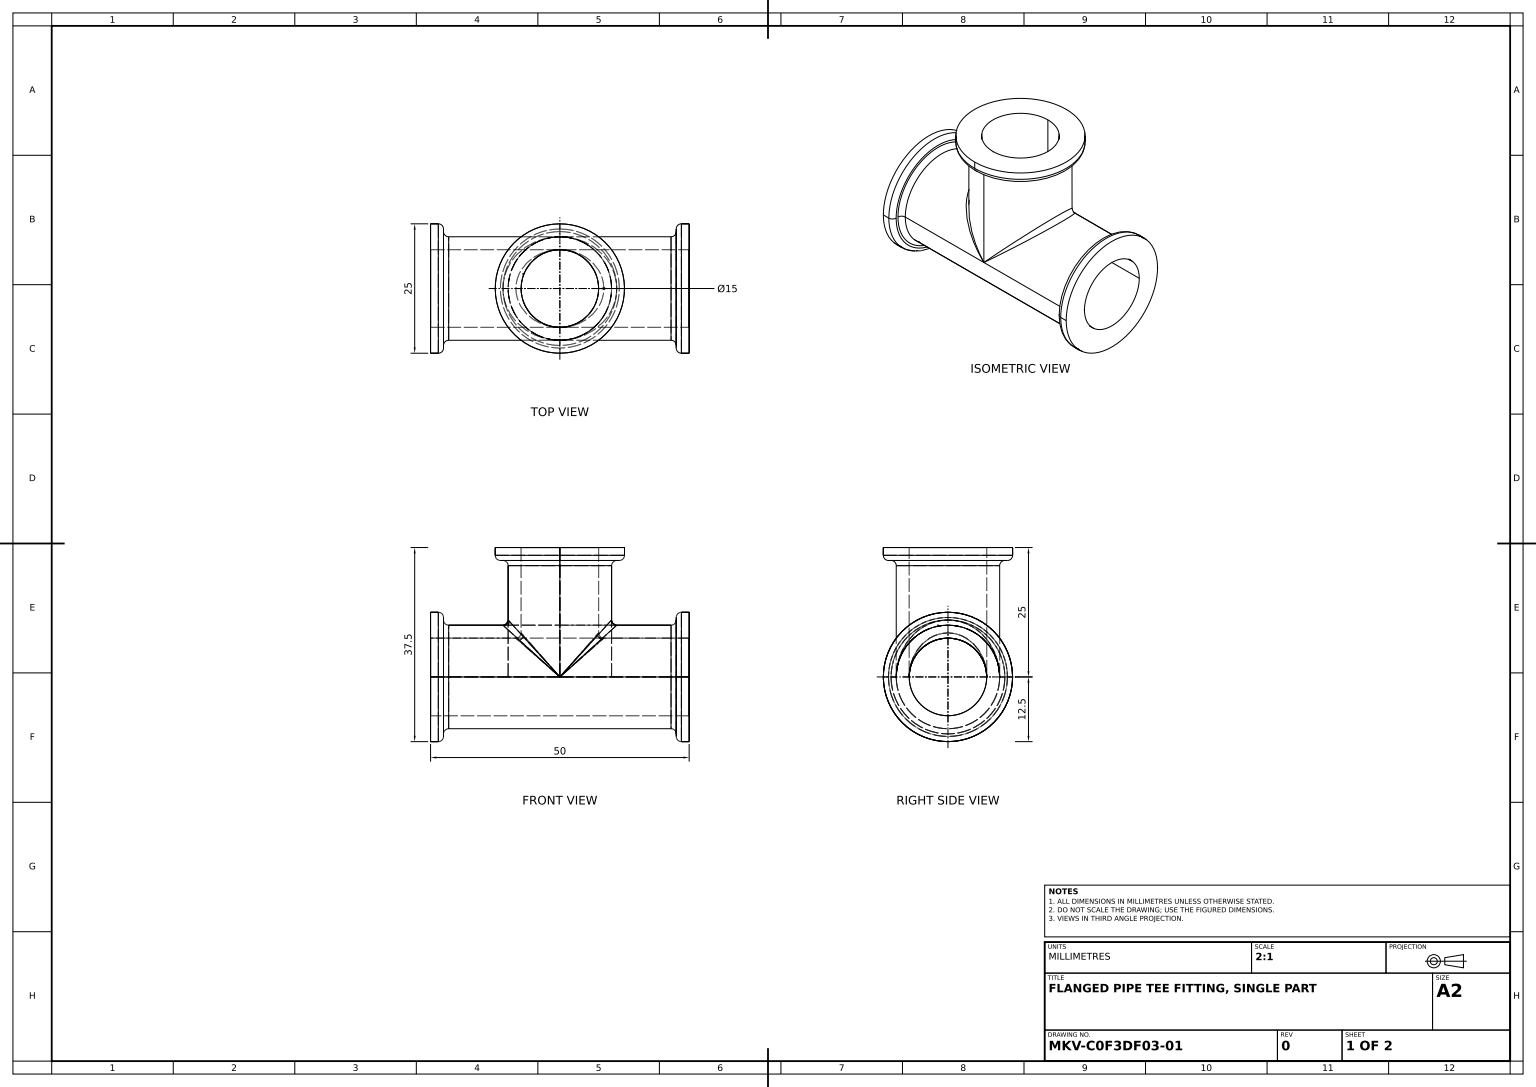
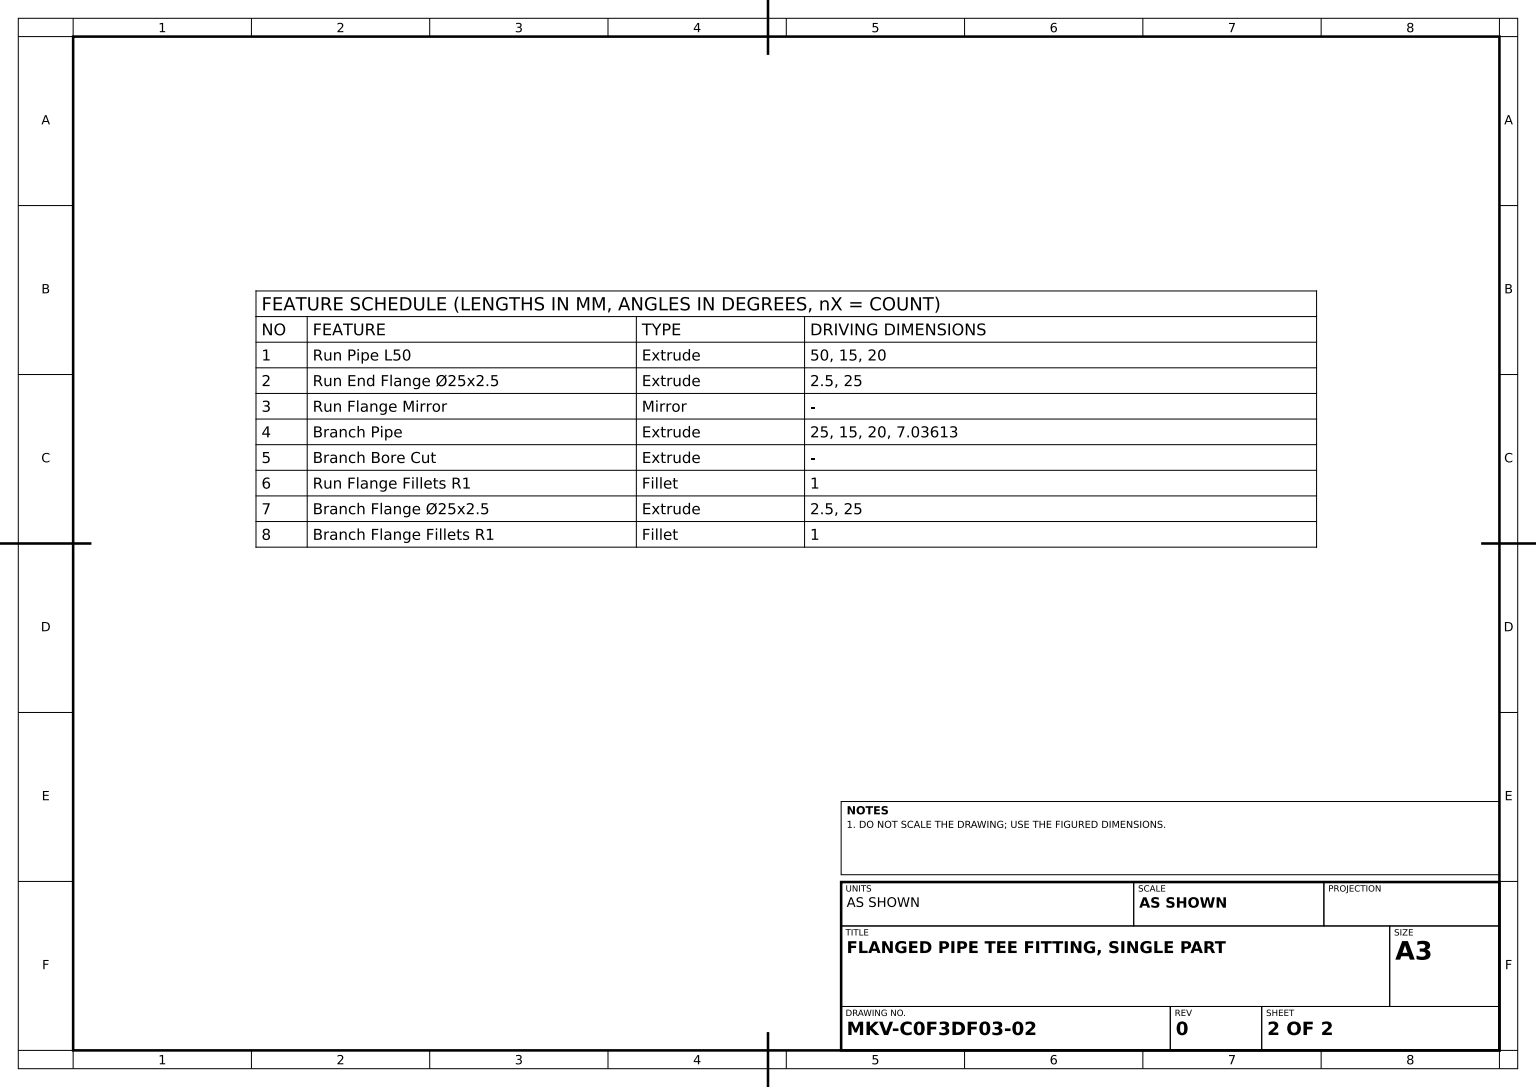
SolidWorks part; units mm, degrees
material "Plain Carbon Steel"
ref_plane "Front Plane" through (0, 0, 0) normal (0, 0, 1) x (1, 0, 0)
ref_plane "Top Plane" through (0, 0, 0) normal (0, 1, 0) x (1, 0, 0)
ref_plane "Right Plane" through (0, 0, 0) normal (1, 0, 0) x (0, 0, -1)
sketch "Run Pipe Profile Ø20-Ø15" plane through (0, 0, 0) normal (1, 0, 0) x (0, 0, -1)
  circle A0 centre (0, 0) radius 7.5
  circle A2 centre (0, 0) radius 10
  dimension "D1" = 15
  dimension "D2" = 20
extrude "Run Pipe L50" add sketch "Run Pipe Profile Ø20-Ø15" against normal blind 50
sketch "Run Flange Profile Ø25" plane through (0, 0, 0) normal (1, 0, 0) x (0, 0, -1)
  circle A0 centre (0, 0) radius 12.5
  circle A1 centre (0, 0) radius 10 construction
  circle A2 centre (0, 0) radius 10
  dimension "D1" = 25
extrude "Run End Flange Ø25x2.5" add sketch "Run Flange Profile Ø25" against normal blind 2.5
ref_plane "Plane1" through (-25, 0, 0) normal (1, 0, 0) x (0, 0, -1)
mirror "Run Flange Mirror" about plane through (-25, 0, 0) normal (1, 0, 0) of "Run End Flange Ø25x2.5"
ref_plane "Plane2" through (0, 25, 0) normal (0, 1, 0) x (1, 0, 0)
sketch "Branch Pipe Profile Ø20-Ø15" plane through (0, 25, 0) normal (0, 1, 0) x (1, 0, 0)
  line L0 (-108.894, 0) -> (8.894, 0) construction
  line L2 (-25, 0) -> (-25, 14.0723) construction
  line L4 (-25, -13.75) -> (-25, 13.75) construction
  circle A0 centre (-25, 0) radius 7.5
  circle A1 centre (-25, 0) radius 10
  point P3 (-50, 0)
  point P7 (-25, 7.0361)
  dimension "D1" = 15
  dimension "D2" = 20
  dimension "D3" = 25
  dimension "D4" = 7.0361
extrude "Branch Pipe" add sketch "Branch Pipe Profile Ø20-Ø15" against normal up to surface (18.3856 mm away)
sketch "Branch Bore Profile" plane through (0, 25, 0) normal (0, 1, 0) x (1, 0, 0)
  circle A2 centre (-25, 0) radius 7.5 construction
  circle A3 centre (-25, 0) radius 7.5
extrude "Branch Bore Cut" cut sketch "Branch Bore Profile" against normal up to surface (25 mm away) up to face at (-50, 0, -7.5)
fillet "Run Flange Fillets R1" radius 1 8 edges at (-2.5, 0, -12.5) (-2.5, 0, -10) (-47.5, 0, -12.5) (-47.5, 0, -10) (-35, 10, 0) (-15, 10, 0) (-17.5, 7.5, 0) (-32.5, 7.5, 0)
sketch "Branch Flange Profile Ø25" plane through (0, 25, 0) normal (0, 1, 0) x (1, 0, 0)
  circle A0 centre (-25, 0) radius 12.5
  circle A1 centre (-25, 0) radius 10 construction
  circle A2 centre (-25, 0) radius 10
  dimension "D1" = 25
extrude "Branch Flange Ø25x2.5" add sketch "Branch Flange Profile Ø25" against normal blind 2.5
fillet "Branch Flange Fillets R1" radius 1 2 edges at (-25, 22.5, 10) (-25, 22.5, 12.5)
